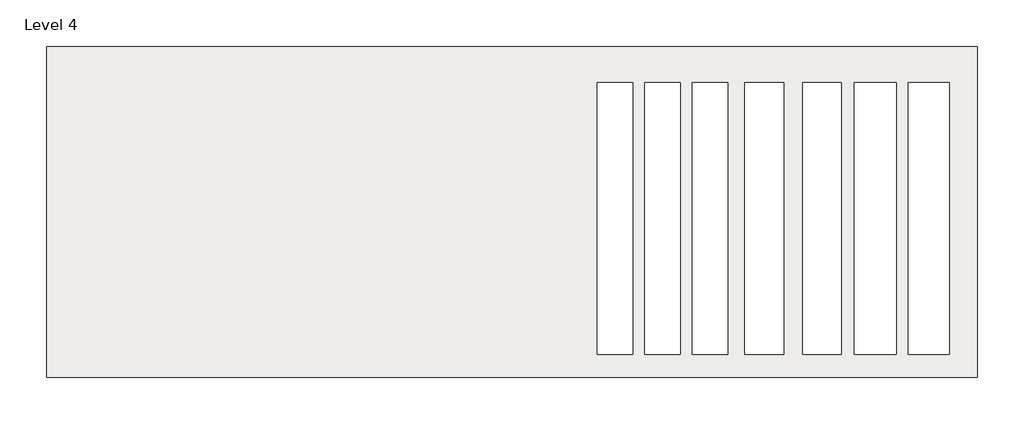
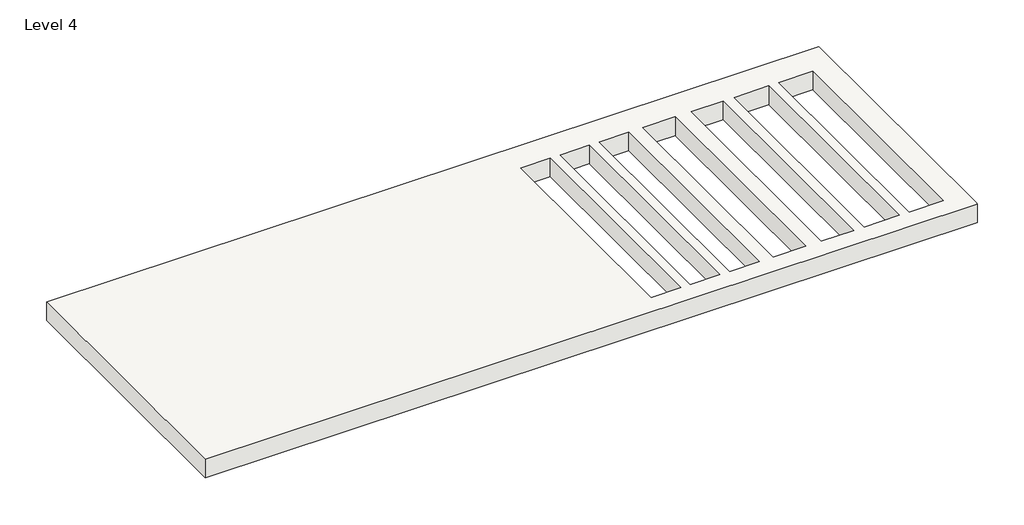
# One storey: 1 roof.
"""IFC4 building model written with IfcOpenShell, lengths in millimetres."""

from ifc_helpers import new_model, si_unit, frame, origin, place, context, project, spatial, polyline, outline, extrude, element, save

model = new_model("IFC4")

# Units and contexts
model_context = context("Model", 3, world=origin())
ifc_project = project(units=[si_unit("LENGTHUNIT", "METRE", prefix="MILLI")], contexts=[model_context])

# Site, building, storey
site = spatial("IfcSite", under=ifc_project)
building = spatial("IfcBuilding", under=site)
storey = spatial("IfcBuildingStorey", under=building, Name="Level 4", Elevation=10972.8)

# Roof
placement = place(None, origin())
element("IfcRoof", 1, ObjectType="Generic - 12\"", at=placement, inside=storey, context=model_context, shape_type="SweptSolid", body=[
    extrude(outline(polyline([(-8374.0311901, 224.6860488), (3614.7688099, 224.6860488), (3614.7688099, -4017.1139512), (3614.7688099, -4042.5139512), (-8374.0311901, -4042.5139512), (-8374.0311901, 224.6860488)]), holes=[polyline([(-823.0035148, -3745.5067029), (-823.0035148, -240.3067029), (-1280.2035148, -240.3067029), (-1280.2035148, -3745.5067029), (-823.0035148, -3745.5067029)]), polyline([(-213.4035148, -3745.5067029), (-213.4035148, -240.3067029), (-670.6035148, -240.3067029), (-670.6035148, -3745.5067029), (-213.4035148, -3745.5067029)]), polyline([(396.1964852, -3745.5067029), (396.1964852, -240.3067029), (-61.0035148, -240.3067029), (-61.0035148, -3745.5067029), (396.1964852, -3745.5067029)]), polyline([(1118.9830783, -3745.5067029), (1118.9830783, -240.3067029), (615.1538938, -240.3067029), (615.1538938, -3745.5067029), (1118.9830783, -3745.5067029)]), polyline([(1862.7309222, -3745.5067029), (1862.7309222, -240.3067029), (1363.1261398, -240.3067029), (1363.1261398, -3745.5067029), (1862.7309222, -3745.5067029)]), polyline([(2570.4909672, -3745.5067029), (2570.4909672, -240.3067029), (2030.6739837, -240.3067029), (2030.6739837, -3745.5067029), (2570.4909672, -3745.5067029)]), polyline([(3254.2591462, -3745.5067029), (3254.2591462, -240.3067029), (2726.4380957, -240.3067029), (2726.4380957, -3745.5067029), (3254.2591462, -3745.5067029)])]), frame((0.0, 0.0, 10972.8), z_axis=(0.0, 0.0, 1.0), x_axis=(1.0, 0.0, 0.0)), (0.0, 0.0, 1.0), 304.8),
])

save(model, "model.ifc")

# Revit data of these elements
# Type "Generic - 12\""
#   Assembly Code = "B1020"
#   Layers, outside or top first: 1' - 0" no material (function 1)
# Element 1 (IfcRoof, "Generic - 12\"")
#   built-in parameter 1001705 = 37 (stored number, unit not read)
#   built-in parameter 1001710 = 33615
#   Phase Created = New Construction
#   Materials on its faces: "Default Roof"
# Materials
#   "Default Roof": colour RGB 88 101 114, transparency 0
